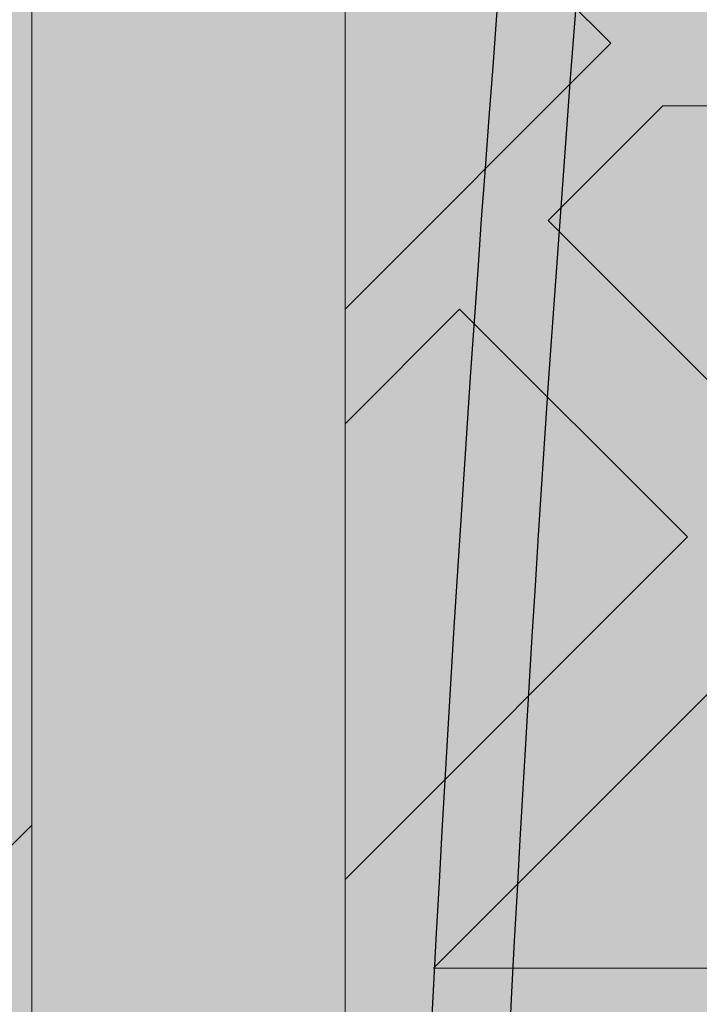
# Model space of a CAD drawing. Units: inches. Extents: x 844 to 2234, y 346 to 1084.
# Tile 78 of 93: x 1998.732 to 2000.116, y 704.51 to 706.514. Entities that reach past the tile are written whole.
import ezdxf

# ---------------------------------------------------------------- set-up
doc = ezdxf.new("R2010")
doc.units = ezdxf.units.IN
doc.header["$MEASUREMENT"] = 0
for name, color, linetype, lineweight in [('A-ANNO-DIMS', 2, 'Continuous', 18), ('furniture', 8, 'Continuous', 18), ('RA-AP-01$0$INT', 35, 'Continuous', 5)]:
    doc.layers.add(name, color=color, linetype=linetype, lineweight=lineweight)
doc.layers.add('RA-AP-01$0$FURN', color=3, linetype='Continuous')
doc.layers.add('RA-AP-01$0$WOOD', color=64, linetype='Continuous')
doc.styles.get("Standard").update_dxf_attribs({"font": 'arial.ttf'})
doc.dimstyles.get("Standard").update_dxf_attribs({"dimtxt": 6, "dimasz": 3, "dimexe": 0.18, "dimexo": 0.0625, "dimgap": 0.09, "dimtad": 0, "dimtih": 1, "dimtoh": 1, "dimdec": 1, "dimzin": 0, "dimdsep": 46, "dimlunit": 3, "dimtxsty": 'Standard', "dimblk": 'ARCHTICK', "dimcen": 0.09, "dimadec": 0, "dimazin": 0, "dimtfac": 1, "dimtdec": 1, "dimtofl": 0, "dimtmove": 0, "dimatfit": 3, "dimfxl": 1, "dimtolj": 1, "dimtzin": 0, "dimarcsym": 0})

# ---------------------------------------------------------------- blocks, each defined once
blk = doc.blocks.new('A$C18D01794')
at = {"layer": 'RA-AP-01$0$INT'}
h = blk.add_hatch(color=256, dxfattribs=at)
h.paths.add_polyline_path([(4.505206456958071, -7.585498806127123), (4.46934859260189, -7.549640941759413), (4.505206456958071, -7.513783077414768), (4.505206456958071, -7.381963272220687), (4.469348592616735, -7.346105407867824), (4.505206456958071, -7.310247543514964), (4.505206456958071, -7.178427738324996), (4.469348592586679, -7.142569873965138), (4.505206456952245, -7.106712009588038), (4.476922185709333, -7.106712009588038), (4.455206456960671, -7.128427738343681), (4.433490728198047, -7.106712009588038), (4.405206456946033, -7.106712009588036), (4.441064321339216, -7.142569873969684), (4.40520645695807, -7.178427738362358), (4.405206456958072, -7.310247543472698), (4.441064321364728, -7.346105407867826), (4.40520645695807, -7.381963272262947), (4.40520645695807, -7.513783077378263), (4.441064321354429, -7.549640941786153), (4.405206456958072, -7.585498806170974), (4.405206456958072, -7.717318611286652), (4.441064321333084, -7.753176475673194), (4.405206456958072, -7.789034340036673), (4.405206456958072, -8.006712009588039), (4.644348592588106, -8.006712009588039), (4.680206456964639, -7.970854145211967), (4.716064321341165, -8.006712009588039), (4.869348592586113, -8.006712009588039), (4.905206456964143, -7.970854145210465), (4.941064321342174, -8.006712009588039), (5.094348592587118, -8.006712009588037), (5.130206456963649, -7.970854145211967), (5.166064321340178, -8.006712009588039), (5.405206456958072, -8.006712009588039), (5.405206456958072, -7.789034340024526), (5.369348592595202, -7.753176475673196), (5.40520645695807, -7.717318611298797), (5.40520645695807, -7.585498806158829), (5.369348592573859, -7.549640941786151), (5.40520645695807, -7.51378307739041), (5.40520645695807, -7.381963272250803), (5.36934859256356, -7.346105407867824), (5.405206456958072, -7.310247543484846), (5.405206456958072, -7.178427738350217), (5.369348592589068, -7.142569873969682), (5.405206456982249, -7.106712009588038), (5.376922185730244, -7.106712009588038), (5.355206456967613, -7.128427738343679), (5.333490728218955, -7.10671200958804), (5.305206456976043, -7.106712009588042), (5.341064321341609, -7.142569873965136), (5.305206456958072, -7.178427738337141), (5.305206456958072, -7.310247543502816), (5.34106432131155, -7.346105407867824), (5.305206456958072, -7.381963272232832), (5.30520645695807, -7.513783077402624), (5.341064321326395, -7.549640941759413), (5.305206456958072, -7.585498806139263), (5.305206456958072, -7.717318611299605), (5.341064321347738, -7.753176475677737), (5.305206456958072, -7.78903434007894), (5.30520645695807, -7.906712009588039), (5.166064321336834, -7.906712009588039), (5.130206456963647, -7.942569873961684), (5.094348592590464, -7.906712009588039), (4.941064321338827, -7.906712009588041), (4.905206456964145, -7.942569873963183), (4.869348592589459, -7.906712009588039), (4.716064321337822, -7.906712009588041), (4.680206456964641, -7.942569873961684), (4.644348592591453, -7.906712009588039), (4.505206456958071, -7.906712009588039), (4.505206456958071, -7.789034340066795), (4.469348592580545, -7.753176475677738), (4.505206456958071, -7.717318611311748)])
h.paths.add_polyline_path([(4.485206456974132, -7.709034340046354), (4.45520645695909, -7.739034340051736), (4.425206456974128, -7.709034340057131), (4.425206456993394, -7.593783077384998), (4.45520645699153, -7.563783077396511), (4.485206456993396, -7.593783077408017)], flags=16)
h.paths.add_polyline_path([(4.455206456954537, -7.767318611299197), (4.485206456958242, -7.797318611312542), (4.48520645695951, -7.912569873958716), (4.45520645695415, -7.942569873954422), (4.425206456957888, -7.912569873967813), (4.425206456957888, -7.797318611286197)], flags=16)
h.paths.add_polyline_path([(4.455206456964794, -7.535498806149051), (4.42520645696469, -7.5054988061393), (4.425206456983954, -7.390247543486406), (4.455206456990734, -7.360247543489279), (4.485206456983953, -7.39024754349214), (4.485206456964687, -7.505498806158811)], flags=16)
h.paths.add_polyline_path([(4.499348592588947, -7.926712009585049), (4.636064321340932, -7.926712009585049), (4.666064321342317, -7.956712009586821), (4.636064321343707, -7.986712009585048), (4.499348592575121, -7.986712009585048), (4.469348592591685, -7.956712009591957)], flags=16)
h.paths.add_polyline_path([(4.425206456957888, -7.940854145195974), (4.471064321332215, -7.986712009585049), (4.425206456957888, -7.986712009585049)], flags=16)
h.paths.add_polyline_path([(4.455206456990734, -7.331963272246367), (4.425206456989053, -7.301963272254337), (4.425206456969784, -7.186712009596224), (4.455206456965226, -7.156712009591144), (4.485206456969787, -7.186712009586051), (4.485206456989053, -7.301963272238404)], flags=16)
h.paths.add_polyline_path([(4.72434859258714, -7.926712009586255), (4.861064321340141, -7.926712009586248), (4.891064321340324, -7.956712009586823), (4.861064321340513, -7.986712009586252), (4.724348592586768, -7.986712009586252), (4.694348592586956, -7.956712009586821)], flags=16)
h.paths.add_polyline_path([(4.919348592587961, -7.956712009586821), (4.949348592588145, -7.92671200958625), (5.08606432134115, -7.926712009586253), (5.116064321341327, -7.956712009586823), (5.086064321341519, -7.986712009586252), (4.949348592587774, -7.986712009586252)], flags=16)
h.paths.add_polyline_path([(5.144348592585967, -7.956712009586823), (5.174348592587358, -7.926712009585049), (5.311064321339338, -7.926712009585049), (5.3410643213366, -7.956712009591957), (5.311064321353163, -7.986712009585048), (5.174348592584576, -7.986712009585048)], flags=16)
h.paths.add_polyline_path([(5.32520645693489, -7.593783077408021), (5.355206456936755, -7.563783077396511), (5.385206456934894, -7.593783077384998), (5.38520645695416, -7.709034340057128), (5.355206456969194, -7.739034340051736), (5.325206456954153, -7.709034340046352)], flags=16)
h.paths.add_polyline_path([(5.325206456970042, -7.797318611312542), (5.355206456973747, -7.767318611299197), (5.385206456970398, -7.7973186112862), (5.385206456970398, -7.912569873967816), (5.355206456974136, -7.942569873954422), (5.325206456968778, -7.912569873958716)], flags=16)
h.paths.add_polyline_path([(5.325206456963599, -7.505498806158811), (5.325206456944333, -7.39024754349214), (5.355206456937552, -7.360247543489279), (5.385206456944332, -7.39024754348641), (5.385206456963596, -7.505498806139303), (5.355206456963492, -7.53549880614905)], flags=16)
h.paths.add_polyline_path([(5.32520645693923, -7.301963272238403), (5.3252064569585, -7.186712009586051), (5.355206456963062, -7.156712009591142), (5.3852064569585, -7.186712009596224), (5.385206456939234, -7.301963272254338), (5.355206456937552, -7.331963272246369)], flags=16)
h.paths.add_polyline_path([(5.339348592596071, -7.986712009585048), (5.385206456970398, -7.940854145195972), (5.385206456970396, -7.986712009585048)], flags=16)
h = blk.add_hatch(color=256, dxfattribs=at)
h.paths.add_polyline_path([(4.469348592586677, -7.142569873965136), (4.505206456958073, -7.178427738324996), (4.505206456958071, -7.106712009582215)])
h.paths.add_polyline_path([(4.455206456960671, -7.128427738343681), (4.476922185709333, -7.106712009588038), (4.433490728198045, -7.106712009588038)])
h.paths.add_polyline_path([(4.405206456958073, -7.178427738362358), (4.441064321339218, -7.142569873969684), (4.40520645695807, -7.106712009600073)])
h.paths.add_polyline_path([(4.425206456989053, -7.301963272254335), (4.455206456990736, -7.331963272246371), (4.485206456989055, -7.301963272238399), (4.48520645696979, -7.186712009586054), (4.455206456965227, -7.15671200959114), (4.425206456969784, -7.186712009596224)])
h.paths.add_polyline_path([(4.505206456958073, -7.381963272220689), (4.505206456958071, -7.310247543514961), (4.469348592616738, -7.346105407867826)])
h.paths.add_polyline_path([(4.425206456964688, -7.5054988061393), (4.455206456964794, -7.535498806149051), (4.485206456964689, -7.505498806158811), (4.485206456983951, -7.390247543492138), (4.455206456990736, -7.360247543489277), (4.425206456983956, -7.39024754348641)])
h.paths.add_polyline_path([(4.425206456974126, -7.709034340057128), (4.455206456959092, -7.739034340051736), (4.485206456974132, -7.709034340046356), (4.485206456993396, -7.593783077408017), (4.45520645699153, -7.563783077396511), (4.425206456993394, -7.593783077384999)])
h.paths.add_polyline_path([(4.46934859260189, -7.549640941759415), (4.505206456958071, -7.585498806127123), (4.505206456958073, -7.513783077414766)])
h.paths.add_polyline_path([(4.405206456958073, -7.585498806170972), (4.441064321354427, -7.549640941786151), (4.405206456958072, -7.513783077378263)])
h.paths.add_polyline_path([(4.405206456958072, -7.789034340036673), (4.441064321333084, -7.753176475673194), (4.405206456958072, -7.71731861128665)])
h.paths.add_polyline_path([(4.469348592580547, -7.75317647567774), (4.505206456958071, -7.789034340066795), (4.505206456958071, -7.717318611311744)])
h.paths.add_polyline_path([(4.425206456957888, -7.912569873967814), (4.45520645695415, -7.942569873954422), (4.485206456959507, -7.912569873958718), (4.48520645695824, -7.797318611312542), (4.455206456954537, -7.767318611299197), (4.425206456957888, -7.797318611286202)])
h.paths.add_polyline_path([(4.425206456957888, -7.986712009585049), (4.471064321332215, -7.986712009585049), (4.425206456957888, -7.940854145195972)])
h.paths.add_polyline_path([(4.499348592575121, -7.986712009585048), (4.636064321343707, -7.986712009585049), (4.666064321342317, -7.956712009586823), (4.636064321340932, -7.926712009585049), (4.499348592588945, -7.926712009585049), (4.469348592591685, -7.95671200959196)])
h.paths.add_polyline_path([(4.680206456964641, -7.942569873961684), (4.716064321337824, -7.906712009588039), (4.644348592591454, -7.906712009588039)])
h.paths.add_polyline_path([(4.644348592588108, -8.006712009588039), (4.716064321341167, -8.006712009588039), (4.680206456964637, -7.970854145211964)])
h.paths.add_polyline_path([(4.724348592586768, -7.98671200958625), (4.861064321340514, -7.986712009586252), (4.891064321340324, -7.956712009586819), (4.861064321340141, -7.92671200958625), (4.724348592587134, -7.926712009586255), (4.694348592586957, -7.956712009586821)])
h.paths.add_polyline_path([(4.905206456964143, -7.942569873963183), (4.941064321338827, -7.906712009588039), (4.869348592589457, -7.906712009588037)])
h.paths.add_polyline_path([(4.869348592586113, -8.006712009588039), (4.941064321342172, -8.006712009588037), (4.905206456964145, -7.970854145210463)])
h.paths.add_polyline_path([(4.949348592587774, -7.986712009586252), (5.086064321341521, -7.986712009586252), (5.116064321341329, -7.956712009586823), (5.08606432134115, -7.926712009586253), (4.949348592588145, -7.92671200958625), (4.919348592587961, -7.956712009586819)])
h.paths.add_polyline_path([(5.130206456963645, -7.942569873961684), (5.166064321336834, -7.906712009588039), (5.094348592590464, -7.906712009588039)])
h.paths.add_polyline_path([(5.094348592587119, -8.006712009588039), (5.166064321340178, -8.006712009588039), (5.130206456963651, -7.970854145211967)])
h.paths.add_polyline_path([(5.174348592584578, -7.986712009585048), (5.311064321353163, -7.986712009585048), (5.341064321336602, -7.956712009591958), (5.31106432133934, -7.926712009585049), (5.174348592587352, -7.926712009585049), (5.144348592585969, -7.956712009586823)])
h.paths.add_polyline_path([(5.325206456968778, -7.912569873958718), (5.355206456974136, -7.942569873954422), (5.385206456970396, -7.912569873967814), (5.385206456970396, -7.797318611286199), (5.355206456973747, -7.767318611299197), (5.325206456970044, -7.797318611312544)])
h.paths.add_polyline_path([(5.339348592596073, -7.986712009585048), (5.385206456970396, -7.986712009585049), (5.385206456970398, -7.94085414519597)])
h.paths.add_polyline_path([(5.325206456954155, -7.709034340046354), (5.355206456969194, -7.739034340051734), (5.38520645695416, -7.709034340057128), (5.385206456934896, -7.593783077384999), (5.355206456936758, -7.563783077396513), (5.325206456934888, -7.593783077408019)])
h.paths.add_polyline_path([(5.305206456958072, -7.789034340078938), (5.341064321347739, -7.753176475677738), (5.305206456958072, -7.717318611299605)])
h.paths.add_polyline_path([(5.369348592595204, -7.753176475673194), (5.40520645695807, -7.789034340024526), (5.405206456958072, -7.717318611298798)])
h.paths.add_polyline_path([(5.405206456958072, -7.585498806158831), (5.405206456958072, -7.513783077390407), (5.369348592573857, -7.549640941786151)])
h.paths.add_polyline_path([(5.305206456958072, -7.585498806139266), (5.341064321326393, -7.549640941759413), (5.305206456958072, -7.513783077402626)])
h.paths.add_polyline_path([(5.325206456963599, -7.50549880615881), (5.355206456963494, -7.535498806149055), (5.385206456963598, -7.505498806139302), (5.385206456944334, -7.390247543486411), (5.355206456937552, -7.360247543489279), (5.325206456944333, -7.39024754349214)])
h.paths.add_polyline_path([(5.305206456958072, -7.38196327223283), (5.341064321311551, -7.346105407867824), (5.305206456958072, -7.31024754350282)])
h.paths.add_polyline_path([(5.325206456939231, -7.301963272238404), (5.355206456937552, -7.331963272246369), (5.385206456939235, -7.301963272254335), (5.385206456958502, -7.186712009596224), (5.355206456963061, -7.156712009591142), (5.3252064569585, -7.186712009586051)])
h.paths.add_polyline_path([(5.404581768715993, -7.381338584008926, -0.001217816984214), (5.405206456958072, -7.381112009582329), (5.405206456958072, -7.310247543484846), (5.369348592563558, -7.346105407867826)])
h.paths.add_polyline_path([(5.36934859258907, -7.142569873969684), (5.40520645695807, -7.178427738350215), (5.405206456958072, -7.106712009612218)])
h.paths.add_polyline_path([(5.355206456967613, -7.128427738343683), (5.376922185730239, -7.106712009588038), (5.333490728218953, -7.10671200958804)])
h.paths.add_polyline_path([(5.30520645695807, -7.178427738337139), (5.341064321341609, -7.142569873965134), (5.305206456958074, -7.10671200957007)])
blk.add_hatch(color=256, dxfattribs=at).paths.add_polyline_path([(4.505206456958071, -7.906712009588039), (5.305206456958072, -7.906712009588039), (5.305206456958072, -7.106712009588038), (5.255206456951893, -7.106712009588036), (5.25520645694868, -7.856712009570104), (4.555206456959269, -7.856712009588616), (4.555206456956052, -7.106712009588038), (4.505206456958073, -7.106712009588038)])
h = blk.add_hatch(color=256, dxfattribs=at)
h.paths.add_polyline_path([(4.585917135068448, -7.856712009587804), (4.614201406330596, -7.856712009587056), (4.668846067270487, -7.802067348644738), (4.723490728212344, -7.856712009584164), (4.771774999457151, -7.856712009582887), (4.826419660396886, -7.80206734864072), (4.862780050090322, -7.838427738332541), (4.844495778842715, -7.856712009580965), (4.862780050090411, -7.856712009580482), (4.905206456960182, -7.814285602707865), (4.947632863832445, -7.856712009578238), (4.965917135079675, -7.856712009577755), (4.947632863831759, -7.838427738330656), (4.983993253523576, -7.802067348637219), (5.038637914464627, -7.856712009575829), (5.08692218571208, -7.856712009574554), (5.141566846649976, -7.802067348634224), (5.196211507589851, -7.856712009571666), (5.224495778822615, -7.856712009570916), (4.905206456953975, -7.537422687702283)])
h.paths.add_polyline_path([(4.895206456956031, -7.575706958950402), (4.895206456958921, -7.684996280828174), (4.840561796018589, -7.630351619890275)], flags=16)
h.paths.add_polyline_path([(4.915206456955638, -7.575706958949956), (4.969851117895509, -7.630351619887399), (4.915206456957609, -7.684996280827732)], flags=16)
h.paths.add_polyline_path([(4.826419660395175, -7.644493755514321), (4.881064321335613, -7.699138416452331), (4.771774999456703, -7.69913841645522)], flags=16)
h.paths.add_polyline_path([(4.983993253519558, -7.644493755510815), (5.038637914460456, -7.699138416449285), (4.929348592581548, -7.69913841645126)], flags=16)
h.paths.add_polyline_path([(4.881064321336025, -7.719138416452334), (4.826419660397532, -7.773783077393256), (4.771774999457062, -7.719138416455217)], flags=16)
h.paths.add_polyline_path([(4.929348592582019, -7.71913841645126), (5.038637914460982, -7.719138416449284), (4.983993253522945, -7.773783077389749)], flags=16)
h.paths.add_polyline_path([(4.895206456960191, -7.733280552075633), (4.895206456962115, -7.806001331460164), (4.876922185715016, -7.824285602708492), (4.840561796021581, -7.787925213016675)], flags=16)
h.paths.add_polyline_path([(4.915206456958487, -7.733280552075187), (4.969851117899527, -7.787925213013798), (4.933490728206909, -7.824285602708034), (4.9152064569598, -7.806001331461736)], flags=16)
h.paths.add_polyline_path([(4.757632863832376, -7.733280552079264), (4.812277524772842, -7.787925213017304), (4.757632863834348, -7.842569873958233)], flags=16)
h.paths.add_polyline_path([(4.737632863832376, -7.73328055207979), (4.737632863834348, -7.842569873958701), (4.682988202893906, -7.787925213020692)], flags=16)
h.paths.add_polyline_path([(5.05278005008503, -7.733280552072701), (5.052780050087917, -7.842569873951664), (4.998135389146995, -7.787925213013169)], flags=16)
h.paths.add_polyline_path([(5.072780050085024, -7.733280552072333), (5.127424711025931, -7.787925213010806), (5.072780050087916, -7.842569873951244)], flags=16)
h.paths.add_polyline_path([(4.935917135072783, -7.506712009583784), (5.255206456948811, -7.826001331459767), (5.255206456948932, -7.797717060211899), (5.200561796010279, -7.743072399273238), (5.255206456949403, -7.688427738334128), (5.25520645694961, -7.640143467086677), (5.200561796009787, -7.585498806146837), (5.236922185702417, -7.549138416454212), (5.255206456949919, -7.56742268770172), (5.255206456949998, -7.549138416454178), (5.212780050078687, -7.506712009583814), (5.25520645695036, -7.464285602712145), (5.255206456950438, -7.446001331464763), (5.236922185702424, -7.464285602712779), (5.200561796009796, -7.427925213020149), (5.255206456950753, -7.373280552079203), (5.25520645695096, -7.324996280834394), (5.200561796010322, -7.270351619893748), (5.255206456951428, -7.215706958952649), (5.255206456951547, -7.187422687705071)])
h.paths.add_polyline_path([(5.042988202883395, -7.42792521302065), (5.097632863823085, -7.373280552080975), (5.097632863822622, -7.482569873959883)], flags=16)
h.paths.add_polyline_path([(5.028846067259663, -7.442067348644384), (5.083490728198774, -7.496712009583504), (4.974201406321001, -7.496712009583035)], flags=16)
h.paths.add_polyline_path([(5.117632863823087, -7.37328055208089), (5.172277524762331, -7.42792521302015), (5.11763286382262, -7.482569873959851)], flags=16)
h.paths.add_polyline_path([(5.08349072819877, -7.516712009582191), (5.028846067259652, -7.571356670521302), (4.974201406320998, -7.516712009582638)], flags=16)
h.paths.add_polyline_path([(5.131774999446817, -7.35913841645716), (5.186419660386065, -7.413783077396415), (5.241064321325782, -7.359138416456712)], flags=17)
h.paths.add_polyline_path([(5.131774999446228, -7.496712009583703), (5.186419660386065, -7.442067348643883), (5.222780050079488, -7.478427738337313), (5.204495778832781, -7.496712009584014)], flags=16)
h.paths.add_polyline_path([(5.097632863822613, -7.530854145205813), (5.097632863823061, -7.640143467084723), (5.042988202883383, -7.585498806145032)], flags=16)
h.paths.add_polyline_path([(5.131774999446899, -7.339138416457162), (5.241064321325809, -7.339138416456712), (5.186419660386591, -7.284493755517479)], flags=17)
h.paths.add_polyline_path([(5.131774999446226, -7.516712009581999), (5.204495778830767, -7.516712009581702), (5.22278005007868, -7.534996280829206), (5.186419660386049, -7.571356670521828)], flags=16)
h.paths.add_polyline_path([(5.11763286382262, -7.530854145205852), (5.17227752476232, -7.585498806145562), (5.117632863823064, -7.64014346708481)], flags=16)
h.paths.add_polyline_path([(5.186419660386069, -7.599640941770585), (5.241064321325754, -7.654285602710281), (5.131774999446791, -7.654285602709814)], flags=16)
h.paths.add_polyline_path([(5.131774999446872, -7.674285602709813), (5.24106432132578, -7.674285602710282), (5.186419660386554, -7.728930263649504)], flags=16)
h.paths.add_polyline_path([(5.255206456951811, -7.126001331467467), (5.255206456951895, -7.106712009588038), (4.555206456956052, -7.106712009588038), (4.555206456956136, -7.12600133146746), (4.905206456953973, -7.476001331465289)])
h.paths.add_polyline_path([(4.983993253513404, -7.368930263651977), (4.92934859257295, -7.314285602713969), (5.03863791445186, -7.314285602711063)], flags=16)
h.paths.add_polyline_path([(4.969851117889988, -7.383072399276016), (4.915206456952556, -7.437717060215906), (4.915206456949648, -7.328427738338133)], flags=16)
h.paths.add_polyline_path([(4.929348592572535, -7.294285602713971), (4.983993253511019, -7.239640941773039), (5.038637914451496, -7.294285602711065)], flags=16)
h.paths.add_polyline_path([(5.052780050074912, -7.280143467087016), (4.998135389134438, -7.225498806148989), (5.052780050072919, -7.170854145208052)], flags=16)
h.paths.add_polyline_path([(5.07278005007491, -7.280143467086489), (5.072780050072918, -7.170854145207579), (5.127424711013374, -7.225498806145578)], flags=16)
h.paths.add_polyline_path([(4.89520645695295, -7.437717060216355), (4.840561796013067, -7.383072399278919), (4.895206456950961, -7.328427738338582)], flags=16)
h.paths.add_polyline_path([(4.915206456948365, -7.280143467090674), (4.915206456946434, -7.207422687704125), (4.933490728192729, -7.18913841645701), (4.969851117886972, -7.225498806149623)], flags=16)
h.paths.add_polyline_path([(4.881064321327021, -7.314285602715054), (4.82641966038902, -7.368930263655506), (4.771774999448108, -7.314285602717047)], flags=16)
h.paths.add_polyline_path([(4.895206456950073, -7.280143467091125), (4.840561796009022, -7.225498806152518), (4.876922185700835, -7.18913841645908), (4.895206456948749, -7.207422687706589)], flags=16)
h.paths.add_polyline_path([(4.983993253510392, -7.211356670525576), (4.947632863816944, -7.174996280833758), (4.965917135064043, -7.156712009585847), (5.038637914448995, -7.156712009584522)], flags=16)
h.paths.add_polyline_path([(4.881064321326543, -7.294285602715056), (4.771774999447578, -7.294285602717046), (4.826419660385607, -7.239640941776569)], flags=16)
h.paths.add_polyline_path([(4.905206456946447, -7.19913841645844), (4.862780050074785, -7.156712009587725), (4.947632863816685, -7.156712009586302)], flags=16)
h.paths.add_polyline_path([(5.14156684663679, -7.211356670521528), (5.086922185696452, -7.156712009583639), (5.196211507574223, -7.156712009581651)], flags=16)
h.paths.add_polyline_path([(4.8264196603837, -7.211356670529104), (4.771774999442643, -7.156712009590501), (4.8444957788276, -7.156712009588568), (4.862780050075511, -7.17499628083566)], flags=16)
h.paths.add_polyline_path([(4.812277524760289, -7.225498806153156), (4.757632863822258, -7.28014346709363), (4.757632863819352, -7.170854145214669)], flags=16)
h.paths.add_polyline_path([(4.73763286382226, -7.280143467093997), (4.682988202881349, -7.22549880615554), (4.737632863819352, -7.170854145215086)], flags=16)
h.paths.add_polyline_path([(4.723490728195188, -7.156712009591787), (4.668846067257299, -7.211356670532127), (4.614201406317417, -7.156712009594693)], flags=16)
h.paths.add_polyline_path([(4.597632863829262, -7.506712009583814), (4.555206456957951, -7.54913841645418), (4.555206456958029, -7.56742268770172), (4.573490728205535, -7.549138416454212), (4.609851117898167, -7.585498806146839), (4.555206456958338, -7.640143467086675), (4.555206456958546, -7.688427738334125), (4.60985111789767, -7.743072399273238), (4.555206456959015, -7.797717060211899), (4.555206456959138, -7.826001331459767), (4.874495778835167, -7.506712009583786), (4.5552064569564, -7.187422687705062), (4.555206456956523, -7.215706958952644), (4.609851117897629, -7.270351619893746), (4.555206456956988, -7.324996280834396), (4.555206456957198, -7.373280552079195), (4.609851117898153, -7.427925213020147), (4.573490728205528, -7.464285602712779), (4.555206456957507, -7.446001331464756), (4.555206456957585, -7.464285602712143)])
h.paths.add_polyline_path([(4.712780050085332, -7.482569873959882), (4.712780050084863, -7.373280552080972), (4.767424711024555, -7.42792521302065)], flags=16)
h.paths.add_polyline_path([(4.726922185709173, -7.496712009583504), (4.781566846648288, -7.442067348644384), (4.836211507586949, -7.496712009583033)], flags=16)
h.paths.add_polyline_path([(4.692780050085327, -7.482569873959851), (4.638135389145619, -7.427925213020149), (4.692780050084865, -7.373280552080892)], flags=16)
h.paths.add_polyline_path([(4.726922185709182, -7.516712009582191), (4.836211507586949, -7.51671200958264), (4.7815668466483, -7.571356670521304)], flags=16)
h.paths.add_polyline_path([(4.678637914461726, -7.496712009583706), (4.605917135075169, -7.496712009584014), (4.587632863828464, -7.478427738337311), (4.623993253521887, -7.442067348643881)], flags=16)
h.paths.add_polyline_path([(4.712780050085336, -7.530854145205816), (4.767424711024568, -7.585498806145034), (4.71278005008489, -7.640143467084724)], flags=16)
h.paths.add_polyline_path([(4.678637914461726, -7.516712009582001), (4.623993253521899, -7.571356670521829), (4.587632863829271, -7.534996280829206), (4.605917135077185, -7.5167120095817)], flags=16)
h.paths.add_polyline_path([(4.692780050085336, -7.530854145205848), (4.692780050084889, -7.64014346708481), (4.638135389145632, -7.585498806145562)], flags=16)
h.paths.add_polyline_path([(4.623993253521885, -7.413783077396415), (4.678637914461131, -7.359138416457161), (4.56934859258217, -7.359138416456712)], flags=17)
h.paths.add_polyline_path([(4.623993253521901, -7.599640941770568), (4.678637914461158, -7.654285602709814), (4.569348592582195, -7.654285602710281)], flags=16)
h.paths.add_polyline_path([(4.678637914461051, -7.339138416457162), (4.623993253521361, -7.284493755517479), (4.569348592582143, -7.339138416456712)], flags=17)
h.paths.add_polyline_path([(4.678637914461076, -7.674285602709813), (4.623993253521399, -7.728930263649504), (4.569348592582167, -7.674285602710281)], flags=16)
h = blk.add_hatch(color=256, dxfattribs=at)
h.paths.add_polyline_path([(5.028846067259997, -7.571356670520955), (4.974201406321342, -7.516712009582294), (5.083490728199115, -7.516712009581846)])
h.paths.add_polyline_path([(4.974201406321344, -7.496712009582688), (5.028846067260004, -7.442067348644037), (5.083490728199117, -7.496712009583157)])
h.paths.add_polyline_path([(5.042988202883738, -7.427925213020309), (5.097632863823428, -7.373280552080627), (5.097632863822963, -7.482569873959537)])
h.paths.add_polyline_path([(5.117632863822961, -7.482569873959509), (5.117632863823428, -7.373280552080546), (5.172277524762674, -7.427925213019804)])
h.paths.add_polyline_path([(5.131774999446572, -7.496712009583358), (5.186419660386406, -7.442067348643536), (5.222780050079831, -7.478427738336961), (5.204495778833122, -7.496712009583667)])
h.paths.add_polyline_path([(5.236922185702764, -7.464285602712433), (5.200561796010139, -7.427925213019802), (5.255206456949971, -7.373280552079975), (5.255206456950271, -7.446001331464927)])
h.paths.add_polyline_path([(5.186419660386412, -7.41378307739607), (5.131774999447164, -7.359138416456815), (5.241064321326123, -7.359138416456366)])
h.paths.add_polyline_path([(5.131774999447238, -7.339138416456815), (5.186419660386934, -7.284493755517132), (5.241064321326153, -7.339138416456368)])
h.paths.add_polyline_path([(5.200561796010663, -7.270351619893402), (5.255206456949324, -7.215706958954747), (5.255206456949777, -7.324996280832518)])
h.paths.add_polyline_path([(5.21278005007903, -7.50671200958347), (5.255206456950223, -7.464285602712278), (5.255206456950696, -7.549138416454185)])
h.paths.add_polyline_path([(5.13177499944657, -7.516712009581652), (5.204495778831106, -7.516712009581354), (5.222780050079024, -7.534996280828858), (5.186419660386397, -7.571356670521485)])
h.paths.add_polyline_path([(5.117632863823405, -7.640143467084465), (5.117632863822955, -7.530854145205498), (5.172277524762665, -7.585498806145217)])
h.paths.add_polyline_path([(5.042988202883727, -7.585498806144689), (5.097632863822957, -7.530854145205474), (5.097632863823407, -7.64014346708438)])
h.paths.add_polyline_path([(5.131774999447135, -7.654285602709467), (5.186419660386394, -7.599640941770219), (5.241064321326097, -7.654285602709933)])
h.paths.add_polyline_path([(5.200561796010128, -7.585498806146492), (5.236922185702758, -7.549138416453866), (5.255206456950264, -7.567422687701371), (5.255206456949948, -7.640143467086325)])
h.paths.add_polyline_path([(5.186419660386895, -7.728930263649157), (5.131774999447213, -7.674285602709467), (5.241064321326127, -7.674285602709934)])
h.paths.add_polyline_path([(5.200561796010624, -7.743072399272893), (5.255206456949745, -7.688427738333778), (5.255206456949276, -7.797717060211553)])
for p, q in [((5.255206456951895, -7.106712009588038), (5.255206456948681, -7.856712009570104)), ((5.305206456940614, -7.381963272250288), (5.34106432131155, -7.346105407867824)), ((5.131774999446817, -7.359138416457161), (5.24106432132578, -7.359138416456712)), ((5.24106432132578, -7.359138416456712), (5.186419660386065, -7.413783077396415)), ((5.255206456949628, -7.373280552080322), (5.200561796009796, -7.427925213020149)), ((5.255206456949927, -7.446001331465273), (5.255206456949628, -7.373280552080322)), ((5.200561796009796, -7.427925213020147), (5.236922185702423, -7.464285602712779)), ((5.186419660386062, -7.442067348643881), (5.222780050078687, -7.478427738336511)), ((5.236922185702423, -7.464285602712779), (5.25520645694988, -7.446001331465319)), ((5.255206456949928, -7.446001331465273), (5.236922185702423, -7.464285602712781)), ((5.212780050078687, -7.506712009583814), (5.25520645694988, -7.464285602712626)), ((5.25520645694988, -7.464285602712626), (5.255206456950353, -7.549138416454534)), ((5.204495778832774, -7.496712009584021), (5.222780050080282, -7.478427738336517)), ((5.204495778831181, -7.496712009584014), (5.131774999446229, -7.496712009583704)), ((5.212780050078687, -7.506712009583814), (5.255206456950353, -7.549138416454534))]:
    blk.add_line(p, q, dxfattribs=at)
blk.add_lwpolyline([(5.305206456958072, -7.106712009588038), (5.305206456958072, -7.906712009588039), (4.505206456958071, -7.906712009588039), (4.505206456958071, -7.106712009588038)], dxfattribs=at)
blk = doc.blocks.new('A$C32926AE1')
at = {"layer": 'RA-AP-01$0$WOOD'}
h = blk.add_hatch(color=256, dxfattribs=at)
h.dxf.hatch_style = 1
h.paths.add_polyline_path([(5.157430609644524, 4.573483066760929, -0.1009492694046607), (5.155401577623758, 4.593365984175333, -0.1842662638101597), (5.172249623284174, 4.638795604568598, 0.2056608120311276), (5.179560981299304, 4.661316324430096, 0.3614336704623542), (5.134352340494423, 4.706524965234944, 0.2056608120311297), (5.111831620632933, 4.699213607219793, -0.1842662638101113), (5.066402000239693, 4.682365561559342, -0.1055311479399994), (5.045656153913092, 4.68467289944697, 0.1567636581983829), (4.763886414745334, 4.684672899446966, -0.1055311479399895), (4.743140568418733, 4.68236556155934, -0.1842662638100833), (4.6977109480255, 4.69921360721979, 0.2056608120302612), (4.675190228164109, 4.706524965234949, 0.3614336704708441), (4.629981587358889, 4.66131632442871, 0.2056608120245944), (4.637292945374126, 4.638795604567974, -0.1842662638101024), (4.654140991034615, 4.59336598417475, -0.1009492694055169), (4.652111959013835, 4.573483066760181, 0.021410119221476), (4.629748025606143, 4.156712009541676, 0.0214101192214795), (4.652111959013809, 3.739940952323101, -0.1009492694059586), (4.654140991034615, 3.720058034908448, -0.1842662638100975), (4.637292945374126, 3.674628414515226, 0.2056608120245705), (4.629981587358889, 3.652107694654492, 0.3614336704708879), (4.675190228164113, 3.606899053848249, 0.2056608120302384), (4.697710948025501, 3.614210411863408, -0.1842662638100995), (4.743140568418738, 3.63105845752386, -0.1055311479402541), (4.763886414745388, 3.628751119636215, 0.1567636581983776), (5.045656153913137, 3.628751119636244, -0.1055311479397538), (5.066402000239692, 3.631058457523857, -0.1842662638101067), (5.111831620632931, 3.614210411863407, 0.2056608120310924), (5.134352340494417, 3.606899053848256, 0.3614336704624001), (5.179560981299307, 3.652107694653103, 0.2056608120311314), (5.172249623284175, 3.6746284145146, -0.1842662638101402), (5.155401577623758, 3.72005803490786, -0.1009492694051366), (5.15743060964455, 3.739940952322354, 0.0214101192215073), (5.179794543052287, 4.156712009541468, 0.0214101192215252)])
h.paths.add_polyline_path([(4.639748609479751, 4.156712009541513, 0.0213537860821624), (4.661970494867118, 3.741887061152232, -0.094075836301374), (4.664143710413708, 3.7196126951003, -0.1824818158568985), (4.644813765429836, 3.668037719127816, 0.2056608120245319), (4.639939526753007, 3.653023905887301, 0.3614336704710246), (4.676106439397173, 3.616856993242342, 0.2056608120302234), (4.691120252638095, 3.621731231919122, -0.1824818158602558), (4.742695228611606, 3.641061176902986, -0.1029891339458722), (4.766991894714349, 3.638256818950944, 0.156709409989566), (5.042550673941472, 3.638256818950105, -0.102989133958497), (5.066847340047078, 3.641061176902949, -0.1824818158594995), (5.118422316020358, 3.621731231919103, 0.2056608120311416), (5.133436129261316, 3.616856993242346, 0.3614336704621468), (5.169603041905217, 3.653023905886178, 0.2056608120310986), (5.164728803228477, 3.668037719127177, -0.1824818158565612), (5.145398858244737, 3.719612695099578, -0.0940758363009313), (5.147572073791232, 3.741887061151398, 0.0213537860822023), (5.169793959178681, 4.156712009541451, 0.0213537860822226), (5.147572073791203, 4.571536957931898, -0.0940758363005034), (5.145398858244737, 4.59381132398362, -0.1824818158565587), (5.164728803228476, 4.645386299956021, 0.2056608120311045), (5.169603041905216, 4.66040011319702, 0.3614336704621845), (5.133436129261313, 4.696567025840856, 0.2056608120310773), (5.118422316020359, 4.691692787164098, -0.182481815859508), (5.066847340047078, 4.67236284218025, -0.1029891339584606), (5.04255067394148, 4.675167200133092, 0.156709409989566), (4.766991894714357, 4.675167200132257, -0.1029891339458842), (4.742695228611611, 4.672362842180213, -0.1824818158602725), (4.691120252638095, 4.691692787164077, 0.2056608120302152), (4.676106439397174, 4.696567025840858, 0.3614336704710363), (4.639939526753005, 4.660400113195899, 0.2056608120245495), (4.644813765429837, 4.645386299955384, -0.1824818158568934), (4.664143710413708, 4.593811323982902, -0.0940758363009187), (4.661970494867149, 4.571536957931074, 0.021353786082177)], flags=16)
h.paths.add_polyline_path([(5.129794543052235, 4.432167055276933, -0.0141661062790638), (5.130152669293814, 4.156927903047693, -0.0141661062790647), (5.129794543052234, 3.881688750818433, -0.0785247771143638), (5.10979738006795, 3.755143611847103, 0.0945969212073497), (5.105408519571111, 3.717898134952927, 0.1043170707844957), (5.116074640131521, 3.670385395016088, 0.1043170707864965), (5.068561900193738, 3.681051515576561, 0.09459692119553), (5.031316423304057, 3.676662655080835, -0.1580239521427272), (4.778226145355827, 3.676662655080367, 0.0945969211986668), (4.740980668464973, 3.681051515576592, 0.1043170707882822), (4.693467928526415, 3.670385395015844, 0.1043170707867916), (4.704134049087309, 3.717898134953662, 0.0945969211972894), (4.69974518859162, 3.755143611844042, -0.0785247771163196), (4.679748025606343, 3.881688750818406, -0.0141661062790663), (4.679389899364763, 4.156927903047693, -0.0141661062790672), (4.679748025606343, 4.432167055276998, -0.0785247771163064), (4.699745188591625, 4.55871219425134, 0.094596921197333), (4.704134049087308, 4.595957671141738, 0.1043170707867205), (4.693467928526416, 4.643470411079523, 0.1043170707882628), (4.740980668464965, 4.632804290518776, 0.0945969211988114), (4.778226145355874, 4.637193151015016, -0.158023952142669), (5.031316423304015, 4.637193151014546, 0.0945969211956361), (5.068561900193736, 4.632804290518806, 0.1043170707864979), (5.11607464013152, 4.643470411079278, 0.1043170707844617), (5.105408519571112, 4.595957671142455, 0.0945969212074597), (5.109797380067959, 4.558712194248236, -0.0785247771143467)], flags=0)
h.paths.add_polyline_path([(5.119794532311105, 4.432259799204851, -0.0142000800617244), (5.120156169157484, 4.156927903047701, -0.0142000800617277), (5.119794532311105, 3.881596006890482, -0.0784894509520253), (5.100273383573699, 3.758192358677797, 0.0940138827242913), (5.095413455884425, 3.717477693979438, 0.0606271852308753), (5.099615656341024, 3.686844378806616, 0.0606271852322524), (5.068982341167493, 3.691046579263239, 0.0940138827010453), (5.028267676478798, 3.686186651576848, -0.1580706864508061), (4.781274892180912, 3.686186651576435, 0.0940138827026903), (4.740560227491556, 3.691046579263279, 0.0606271852339895), (4.709926912317155, 3.686844378806508, 0.0606271852329405), (4.714129112773991, 3.717477693980356, 0.094013882701304), (4.709269185087677, 3.758192358669163, -0.0784894509577193), (4.689748036347473, 3.881596006890469, -0.014200080061729), (4.689386399501094, 4.156927903047709, -0.0142000800617217), (4.689748036347473, 4.432259799204808, -0.078489450957724), (4.709269185087651, 4.555663447426125, 0.0940138827014585), (4.714129112773992, 4.596378112114996, 0.0606271852329731), (4.709926912317154, 4.62701142728886, 0.0606271852340196), (4.74056022749157, 4.622809226832087, 0.0940138827024997), (4.781274892180847, 4.627669154518912, -0.1580706864508359), (5.028267676478777, 4.627669154518526, 0.0940138827010946), (5.068982341167492, 4.622809226832129, 0.060627185232254), (5.099615656341024, 4.627011427288751, 0.0606271852308727), (5.095413455884425, 4.59637811211593, 0.0940138827241088), (5.100273383573675, 4.555663447417647, -0.0784894509520978)], flags=0)
h.paths.add_polyline_path([(5.06978912287499, 4.430218106756144, -0.014241683694547), (5.070173729147532, 4.156927903047672, -0.0142416836945458), (5.06978912287499, 3.883637699339223, -0.0800609523125196), (5.052662118612511, 3.773463122773442, 0.0526421978001116), (5.04590916754064, 3.740550867606997, 0.0526421977992423), (5.012996912374707, 3.73379791653534, -0.1583028414718258), (4.796545656286308, 3.73379791653451, 0.0526421978034211), (4.763633401117837, 3.740550867607021, 0.0526421978018622), (4.756880450045755, 3.773463122774558, -0.0800609523117106), (4.739753445783639, 3.883637699339268, -0.0142416836945435), (4.739368839511098, 4.156927903047671, -0.0142416836945477), (4.739753445783639, 4.430218106756155, -0.0800609523116345), (4.75688045004574, 4.540392683320762, 0.052642197801941), (4.763633401117837, 4.573304938488346, 0.0526421978035071), (4.796545656286361, 4.580057889560873, -0.1583028414717561), (5.012996912374669, 4.580057889560039, 0.0526421977993048), (5.04590916754064, 4.57330493848837, 0.0526421978002057), (5.052662118612529, 4.540392683321868, -0.080060952312477)], flags=0)
h.paths.add_polyline_path([(5.049789715110557, 4.43038092723357, -0.0143097550741839), (5.05018085590259, 4.156927903047715, -0.0143097550741854), (5.049789715110558, 3.883474878861827, -0.0800685599149176), (5.03362098255317, 3.779581877367999, 0.0306258898956367), (5.028241146483733, 3.758218888663947, 0.0306258898977031), (5.006878157778253, 3.75283905259408, -0.1583983521624096), (4.802664410878162, 3.752839052594731, 0.0306258898946014), (4.781301422174808, 3.758218888663924, 0.0306258898967912), (4.775921586105202, 3.779581877368794, -0.080068559914251), (4.759752853548071, 3.883474878861786, -0.0143097550741854), (4.759361712756037, 4.156927903047671, -0.0143097550741854), (4.759752853548071, 4.430380927233557, -0.0800685599142479), (4.775921586105193, 4.534273928726546, 0.0306258898968306), (4.781301422174808, 4.555636917431444, 0.0306258898945754), (4.802664410878143, 4.561016753500631, -0.1583983521624168), (5.006878157778244, 4.561016753501291, 0.0306258898977177), (5.028241146483733, 4.555636917431421, 0.0306258898958182), (5.03362098255321, 4.534273928727244, -0.080068559914796)], flags=0)
h.paths.add_polyline_path([(4.999766070382627, 4.428171244713864, -0.0143443147609634), (5.000198441819402, 4.156927903047689, -0.0143443147609612), (4.999766070382627, 3.885684561381556, -0.0784641635803329), (4.987356730658798, 3.799103304488872, -0.1506053783831347), (4.822185837999821, 3.79910330448882, -0.0784641635803318), (4.809776498276007, 3.885684561381509, -0.014344314760963), (4.809344126839227, 4.156927903047677, -0.0143443147609645), (4.809776498276007, 4.428171244713873, -0.0784641635803192), (4.822185837999822, 4.514752501606549, -0.1506053783831338), (4.987356730658798, 4.514752501606494, -0.078464163580285)], flags=0)
h.paths.add_polyline_path([(4.979755254238824, 4.42764379880488, -0.0143772539198268), (4.980205517789977, 4.156927903047693, -0.0143772539198275), (4.979755254238824, 3.886212007290489, -0.0689242507424422), (4.971183264704897, 3.815276770442801, -0.1296645318904179), (4.838359303953726, 3.815276770442746, -0.0689242507424186), (4.829787314419809, 3.886212007290419, -0.0143772539198292), (4.829337050868653, 4.156927903047653, -0.0143772539198325), (4.829787314419809, 4.427643798804946, -0.0689242507424211), (4.838359303953725, 4.498579035652621, -0.1296645318904187), (4.971183264704897, 4.498579035652565, -0.0689242507424401)], flags=0)
h = blk.add_hatch(color=256, dxfattribs=at)
h.dxf.hatch_style = 1
h.paths.add_polyline_path([(5.145398858244737, 4.59381132398362, -0.1824818158565616), (5.164728803228476, 4.645386299956021, 0.2056608120311045), (5.169603041905216, 4.66040011319702, 0.3614336704621845), (5.133436129261313, 4.696567025840856, 0.2056608120310773), (5.118422316020359, 4.691692787164098, -0.182481815859508), (5.066847340047078, 4.67236284218025, -0.1029891339584606), (5.04255067394148, 4.675167200133092, 0.156709409989566), (4.766991894714357, 4.675167200132257, -0.1029891339458842), (4.742695228611611, 4.672362842180213, -0.1824818158602725), (4.691120252638095, 4.691692787164077, 0.2056608120302152), (4.676106439397174, 4.696567025840858, 0.3614336704710363), (4.639939526753005, 4.660400113195899, 0.2056608120245495), (4.644813765429837, 4.645386299955384, -0.1824818158568934), (4.664143710413708, 4.593811323982902, -0.0940758363009187), (4.661970494867149, 4.571536957931074, 0.0213537860821772), (4.639748609479751, 4.156712009541507, 0.0213537860821625), (4.661970494867119, 3.741887061152226, -0.0940758363013071), (4.664143710413708, 3.719612695100309, -0.1824818158569294), (4.644813765429836, 3.668037719127816, 0.2056608120245319), (4.639939526753007, 3.653023905887301, 0.3614336704710246), (4.676106439397173, 3.616856993242342, 0.2056608120302234), (4.691120252638095, 3.621731231919122, -0.1824818158602558), (4.742695228611606, 3.641061176902986, -0.1029891339458722), (4.766991894714349, 3.638256818950944, 0.156709409989566), (5.042550673941472, 3.638256818950105, -0.102989133958497), (5.066847340047078, 3.641061176902949, -0.1824818158594995), (5.118422316020358, 3.621731231919103, 0.2056608120311416), (5.133436129261316, 3.616856993242346, 0.3614336704621468), (5.169603041905217, 3.653023905886178, 0.2056608120310986), (5.164728803228477, 3.668037719127177, -0.1824818158565612), (5.145398858244737, 3.719612695099578, -0.0940758363009313), (5.147572073791232, 3.741887061151398, 0.0213537860822023), (5.169793959178681, 4.156712009541451, 0.0213537860822226), (5.147572073791203, 4.571536957931898, -0.0940758363004996)])
h.paths.add_polyline_path([(5.109797380067958, 4.55871219424824, -0.0785247771143472), (5.129794543052234, 4.432167055276936, -0.0141661062790644), (5.130152669293814, 4.156927903047685, -0.014166106279066), (5.129794543052234, 3.881688750818401, -0.0785247771143517), (5.109797380067946, 3.755143611847092, 0.0945969212073132), (5.105408519571111, 3.717898134952929, 0.1043170707844995), (5.116074640131521, 3.670385395016088, 0.1043170707864965), (5.068561900193738, 3.681051515576561, 0.09459692119553), (5.031316423304057, 3.676662655080835, -0.1580239521427272), (4.778226145355827, 3.676662655080367, 0.0945969211986668), (4.740980668464973, 3.681051515576592, 0.1043170707882822), (4.693467928526415, 3.670385395015844, 0.1043170707867916), (4.704134049087309, 3.717898134953662, 0.0945969211972894), (4.69974518859162, 3.755143611844042, -0.0785247771163196), (4.679748025606343, 3.881688750818406, -0.0141661062790663), (4.679389899364763, 4.156927903047693, -0.0141661062790672), (4.679748025606343, 4.432167055276998, -0.0785247771163064), (4.699745188591625, 4.55871219425134, 0.094596921197333), (4.704134049087308, 4.595957671141738, 0.1043170707867205), (4.693467928526416, 4.643470411079523, 0.1043170707882628), (4.740980668464965, 4.632804290518776, 0.0945969211988114), (4.778226145355874, 4.637193151015016, -0.158023952142669), (5.031316423304015, 4.637193151014546, 0.0945969211956361), (5.068561900193736, 4.632804290518806, 0.1043170707864979), (5.11607464013152, 4.643470411079278, 0.1043170707844617), (5.105408519571112, 4.595957671142455, 0.0945969212074504)], flags=16)
h.paths.add_polyline_path([(5.100273383573655, 4.55566344741771, -0.0784894509521388), (5.119794532311105, 4.432259799204852, -0.0142000800617252), (5.120156169157484, 4.156927903047686, -0.014200080061726), (5.119794532311105, 3.881596006890502, -0.0784894509520446), (5.100273383573696, 3.758192358677786, 0.0940138827242721), (5.095413455884425, 3.717477693979436, 0.0606271852308692), (5.099615656341024, 3.686844378806616, 0.0606271852322522), (5.068982341167493, 3.691046579263239, 0.0940138827010453), (5.028267676478798, 3.686186651576848, -0.1580706864508061), (4.781274892180912, 3.686186651576435, 0.0940138827026903), (4.740560227491556, 3.691046579263279, 0.0606271852339895), (4.709926912317155, 3.686844378806508, 0.0606271852329405), (4.714129112773991, 3.717477693980356, 0.094013882701304), (4.709269185087677, 3.758192358669163, -0.0784894509577193), (4.689748036347473, 3.881596006890469, -0.014200080061729), (4.689386399501094, 4.156927903047709, -0.0142000800617217), (4.689748036347473, 4.432259799204808, -0.078489450957724), (4.709269185087651, 4.555663447426125, 0.0940138827014585), (4.714129112773992, 4.596378112114996, 0.0606271852329731), (4.709926912317154, 4.62701142728886, 0.0606271852340196), (4.74056022749157, 4.622809226832087, 0.0940138827024997), (4.781274892180847, 4.627669154518912, -0.1580706864508359), (5.028267676478777, 4.627669154518526, 0.0940138827010946), (5.068982341167492, 4.622809226832129, 0.060627185232254), (5.099615656341024, 4.627011427288751, 0.0606271852308727), (5.095413455884425, 4.59637811211593, 0.094013882723957)], flags=0)
h.paths.add_polyline_path([(5.04590916754064, 4.57330493848837, 0.0526421978002057), (5.052662118612529, 4.540392683321868, -0.0800609523124783), (5.06978912287499, 4.430218106756142, -0.0142416836945469), (5.070173729147532, 4.156927903047672, -0.0142416836945458), (5.06978912287499, 3.883637699339223, -0.0800609523125196), (5.052662118612511, 3.773463122773442, 0.0526421978001116), (5.04590916754064, 3.740550867606997, 0.0526421977992423), (5.012996912374707, 3.73379791653534, -0.1583028414718258), (4.796545656286308, 3.73379791653451, 0.0526421978034211), (4.763633401117837, 3.740550867607021, 0.0526421978018622), (4.756880450045755, 3.773463122774558, -0.0800609523117106), (4.739753445783639, 3.883637699339268, -0.0142416836945435), (4.739368839511098, 4.156927903047671, -0.0142416836945477), (4.739753445783639, 4.430218106756155, -0.0800609523116345), (4.75688045004574, 4.540392683320762, 0.052642197801941), (4.763633401117837, 4.573304938488346, 0.0526421978035071), (4.796545656286361, 4.580057889560873, -0.1583028414717561), (5.012996912374669, 4.580057889560039, 0.0526421977993048)], flags=0)
h.paths.add_polyline_path([(5.028241146483733, 4.555636917431422, 0.0306258898956949), (5.033620982553182, 4.534273928727329, -0.0800685599148649), (5.049789715110557, 4.430380927233569, -0.0143097550741839), (5.05018085590259, 4.156927903047715, -0.0143097550741854), (5.049789715110558, 3.883474878861827, -0.0800685599149176), (5.03362098255317, 3.779581877367999, 0.0306258898956367), (5.028241146483733, 3.758218888663947, 0.0306258898977031), (5.006878157778253, 3.75283905259408, -0.1583983521624096), (4.802664410878162, 3.752839052594731, 0.0306258898946014), (4.781301422174808, 3.758218888663924, 0.0306258898967912), (4.775921586105202, 3.779581877368794, -0.080068559914251), (4.759752853548071, 3.883474878861786, -0.0143097550741854), (4.759361712756037, 4.156927903047671, -0.0143097550741854), (4.759752853548071, 4.430380927233557, -0.0800685599142479), (4.775921586105193, 4.534273928726546, 0.0306258898968306), (4.781301422174808, 4.555636917431444, 0.0306258898945754), (4.802664410878143, 4.561016753500631, -0.1583983521624168), (5.006878157778244, 4.561016753501291, 0.0306258898977174)], flags=0)
h.paths.add_polyline_path([(4.987356730658798, 4.514752501606494, -0.0784641635803018), (4.999766070382627, 4.428171244713845, -0.0143443147609637), (5.000198441819402, 4.156927903047665, -0.0143443147609622), (4.999766070382628, 3.885684561381514, -0.0784641635802952), (4.987356730658797, 3.799103304488872, -0.1506053783831338), (4.822185837999821, 3.799103304488819, -0.0784641635803342), (4.809776498276007, 3.885684561381512, -0.0143443147609628), (4.809344126839227, 4.156927903047676, -0.0143443147609646), (4.809776498276007, 4.428171244713873, -0.0784641635803192), (4.822185837999822, 4.514752501606549, -0.1506053783831338)], flags=0)
h.paths.add_polyline_path([(4.971183264704897, 4.498579035652566, -0.0689242507424384), (4.979755254238824, 4.427643798804883, -0.0143772539198276), (4.980205517789977, 4.15692790304768, -0.0143772539198258), (4.979755254238823, 3.88621200729051, -0.0689242507424628), (4.971183264704897, 3.815276770442801, -0.129664531890417), (4.838359303953726, 3.815276770442746, -0.0689242507424186), (4.829787314419809, 3.886212007290419, -0.0143772539198292), (4.829337050868653, 4.156927903047653, -0.0143772539198325), (4.829787314419809, 4.427643798804946, -0.0689242507424211), (4.838359303953725, 4.498579035652621, -0.1296645318904187)], flags=0)
for radius, end in [(4.875754844654793, 5.524589681839913), (4.865754844654794, 5.512956158076888)]:
    blk.add_arc((0.304323780376417, 4.104079819130551), radius, 0.6185013483537143, end, dxfattribs=at)
blk = doc.blocks.new('A$C5D2F253E')
at = {"layer": 'RA-AP-01$0$FURN', "xscale": -0.7999999999883585, "yscale": 0.7999999999883585, "zscale": 0.8, "rotation": 90}
blk.add_blockref('A$C18D01794', (-5.687757199772477, 4.75791982714071), dxfattribs=at)
at = {"layer": 'RA-AP-01$0$WOOD', "rotation": 270}
blk.add_blockref('A$C32926AE1', (-4.161339601644158, 5.73852594588169), dxfattribs=at)
blk = doc.blocks.new('_ArchTick')
at = {"color": 0, "linetype": 'ByBlock', "const_width": 0.15}
blk.add_lwpolyline([(-0.5, -0.5), (0.5, 0.5)], dxfattribs=at)
blk = doc.blocks.new('*D121')
at = {"layer": 'A-ANNO-DIMS', "color": 0, "lineweight": -2, "transparency": 16777216}
for p, q in [((2030.271987351997, 734.262611118704), (2040.245275089302, 734.262611118704)), ((2040.065275089302, 734.262611118704), (2040.065275089302, 704.6043509484256)), ((2040.065275089302, 668.557359536674), (2040.065275089302, 698.2156197069523)), ((2030.271987351997, 668.557359536674), (2040.245275089302, 668.557359536674))]:
    blk.add_line(p, q, dxfattribs=at)
at = {"layer": 'Defpoints', "color": 0, "transparency": 16777216}
for p in [(2030.209487351997, 734.262611118704), (2040.065275089302, 734.262611118704), (2030.209487351997, 668.557359536674)]:
    blk.add_point(p, dxfattribs=at)
at = {"layer": 'A-ANNO-DIMS', "color": 0, "lineweight": -2, "transparency": 16777216, "xscale": 3, "yscale": 3, "zscale": 3}
for p, rotation in [((2040.065275089302, 734.262611118704), 90), ((2040.065275089302, 668.557359536674), 270)]:
    blk.add_blockref('_ArchTick', p, dxfattribs=dict(at, rotation=rotation))
at = {"layer": 'A-ANNO-DIMS', "color": 0, "transparency": 16777216, "insert": (2040.065275089302, 701.4099853276883), "char_height": 6, "attachment_point": 5}
blk.add_mtext('\\A1;LOUNGE SET 5\'-5 1/2" TYP.', dxfattribs=at)

msp = doc.modelspace()

# ---------------------------------------------------------------- block references
at = {"layer": 'furniture', "xscale": -15.94108302203742, "yscale": 15.94108302203742, "zscale": 15.94108302203742, "rotation": 270}
msp.add_blockref('A$C5D2F253E', (1990.567271852805, 701.4028671565849), dxfattribs=at)

# ---------------------------------------------------------------- dimensions: what is measured, and where the dimension line sits
at = {"layer": 'A-ANNO-DIMS'}
dim = msp.add_linear_dim(base=(2040.065275089302, 734.262611118704), p1=(2030.209487351996, 668.5573595366737), p2=(2030.209487351996, 734.2626111187037), angle=90, text='LOUNGE SET <> TYP.', dimstyle='Standard', override={"dimdec": 1, "dimlfac": 1, "dimrnd": 0, "dimzin": 1, "dimdsep": 46, "dimlunit": 4, "dimfrac": 2}, dxfattribs=at)
dim.commit()
dim.dimension.update_dxf_attribs({"geometry": '*D121', "text_midpoint": (2040.065275089302, 701.4099853276883)})

doc.saveas('drawing.dxf')
